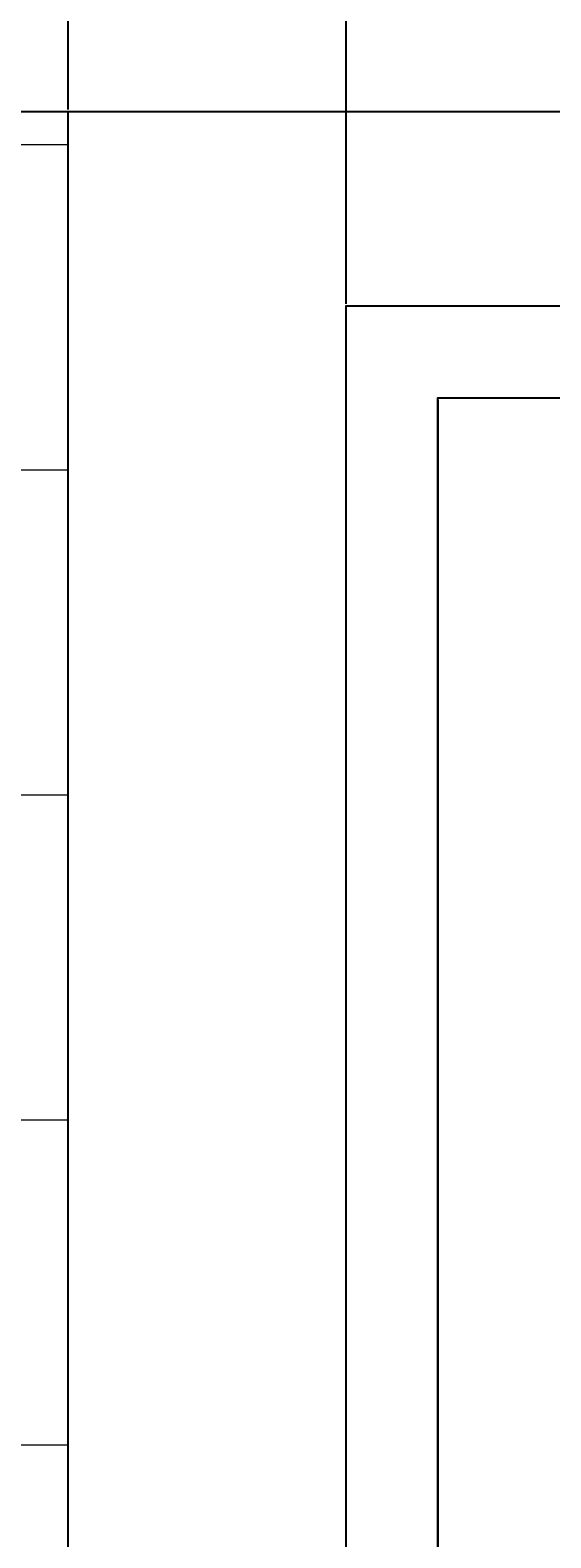
# Model space of a CAD drawing. Units: inches. Extents: x 37 to 824, y -700 to 234.
# Tile 16 of 77: x 298 to 315, y -536 to -487. Entities that reach past the tile are written whole.
import ezdxf

# ---------------------------------------------------------------- set-up
doc = ezdxf.new("R2010")
doc.units = ezdxf.units.IN
doc.header["$MEASUREMENT"] = 0
for name, color, linetype, lineweight in [('A-ANNO-DIMS', 2, 'Continuous', 18), ('A-DOOR', 4, 'Continuous', 25), ('A-ELEV', 3, 'Continuous', 25), ('A-ELEV-PATT', 8, 'Continuous', 13)]:
    doc.layers.add(name, color=color, linetype=linetype, lineweight=lineweight)
doc.styles.get("Standard").update_dxf_attribs({"font": 'arial.ttf'})
doc.dimstyles.get("Standard").update_dxf_attribs({"dimtxt": 0.18, "dimasz": 0.18, "dimexe": 0.18, "dimexo": 0.0625, "dimgap": 0.09, "dimtad": 0, "dimtih": 1, "dimtoh": 1, "dimdec": 1, "dimzin": 0, "dimdsep": 46, "dimlunit": 4, "dimtxsty": 'Standard', "dimcen": 0.09, "dimadec": 0, "dimazin": 0, "dimtfac": 1, "dimtdec": 1, "dimtofl": 0, "dimtmove": 0, "dimatfit": 3, "dimfxl": 1, "dimtolj": 1, "dimtzin": 0, "dimarcsym": 0})

# ---------------------------------------------------------------- blocks, each defined once
blk = doc.blocks.new('*U9')
blk.add_lwpolyline([(3.124, 0.013), (0.124, 0.013), (0.124, 84.013), (40.124, 84.013), (40.124, 0.013), (37.124, 0.013)])
blk.add_lwpolyline([(37.124, 80.99), (37.124, 0.013), (3.124, 0.013), (3.124, 80.99)], close=True)
blk = doc.blocks.new('*D31')
at = {"layer": 'A-ANNO-DIMS', "color": 0, "lineweight": -2, "ltscale": 0.5, "transparency": 16777216}
for p, q in [((255.14, -489.627), (449.772, -489.627)), ((449.592, -495.627), (449.592, -510.537)), ((449.592, -531.627), (449.592, -516.717)), ((255.14, -537.627), (449.772, -537.627))]:
    blk.add_line(p, q, dxfattribs=at)
at = {"layer": 'A-ANNO-DIMS', "color": 0, "ltscale": 0.5, "transparency": 16777216}
for points in [[(448.592, -495.627), (450.592, -495.627), (449.592, -489.627)], [(448.592, -531.627), (450.592, -531.627), (449.592, -537.627)]]:
    blk.add_solid(points, dxfattribs=at)
at = {"layer": 'Defpoints', "color": 0, "ltscale": 0.5, "transparency": 16777216}
for p in [(255.077, -489.627), (449.592, -489.627), (255.077, -537.627)]:
    blk.add_point(p, dxfattribs=at)
at = {"layer": 'A-ANNO-DIMS', "color": 0, "ltscale": 0.5, "transparency": 16777216, "insert": (449.592, -513.627), "char_height": 6, "attachment_point": 5}
blk.add_mtext("\\A1;4'", dxfattribs=at)
blk = doc.blocks.new('*D98')
at = {"layer": 'A-ANNO-DIMS', "color": 0, "lineweight": -2, "ltscale": 0.5, "transparency": 16777216}
for p, q in [((299.077, -489.565), (299.077, -378.38)), ((308.196, -495.944), (308.196, -378.38)), ((299.257, -378.56), (303.307, -378.56)), ((308.016, -378.56), (303.966, -378.56))]:
    blk.add_line(p, q, dxfattribs=at)
at = {"layer": 'A-ANNO-DIMS', "color": 0, "ltscale": 0.5, "transparency": 16777216}
for points in [[(299.257, -378.53), (299.257, -378.59), (299.077, -378.56)], [(308.016, -378.53), (308.016, -378.59), (308.196, -378.56)]]:
    blk.add_solid(points, dxfattribs=at)
at = {"layer": 'Defpoints', "color": 0, "ltscale": 0.5, "transparency": 16777216}
for p in [(308.196, -378.56), (299.077, -489.627), (308.196, -496.007)]:
    blk.add_point(p, dxfattribs=at)
at = {"layer": 'A-ANNO-DIMS', "color": 0, "ltscale": 0.5, "transparency": 16777216, "insert": (303.636, -378.56), "char_height": 0.18, "attachment_point": 5}
blk.add_mtext('\\A1;0\'-9"', dxfattribs=at)
blk = doc.blocks.new('*D99')
at = {"layer": 'A-ANNO-DIMS', "color": 0, "lineweight": -2, "ltscale": 0.5, "transparency": 16777216}
for p, q in [((308.196, -495.944), (308.196, -378.38)), ((348.196, -495.944), (348.196, -378.38)), ((308.376, -378.56), (327.866, -378.56)), ((348.016, -378.56), (328.525, -378.56))]:
    blk.add_line(p, q, dxfattribs=at)
at = {"layer": 'A-ANNO-DIMS', "color": 0, "ltscale": 0.5, "transparency": 16777216}
for points in [[(308.376, -378.53), (308.376, -378.59), (308.196, -378.56)], [(348.016, -378.53), (348.016, -378.59), (348.196, -378.56)]]:
    blk.add_solid(points, dxfattribs=at)
at = {"layer": 'Defpoints', "color": 0, "ltscale": 0.5, "transparency": 16777216}
for p in [(348.196, -378.56), (308.196, -496.007), (348.196, -496.007)]:
    blk.add_point(p, dxfattribs=at)
at = {"layer": 'A-ANNO-DIMS', "color": 0, "ltscale": 0.5, "transparency": 16777216, "insert": (328.196, -378.56), "char_height": 0.18, "attachment_point": 5}
blk.add_mtext('\\A1;3\'-4"', dxfattribs=at)
blk = doc.blocks.new('*D102')
at = {"layer": 'A-ANNO-DIMS', "color": 0, "lineweight": -2, "ltscale": 0.5, "transparency": 16777216}
for p, q in [((311.196, -499.092), (311.196, -699.594)), ((345.196, -499.092), (345.196, -699.594)), ((311.376, -699.414), (327.795, -699.414)), ((345.016, -699.414), (328.596, -699.414))]:
    blk.add_line(p, q, dxfattribs=at)
at = {"layer": 'A-ANNO-DIMS', "color": 0, "ltscale": 0.5, "transparency": 16777216}
for points in [[(311.376, -699.384), (311.376, -699.444), (311.196, -699.414)], [(345.016, -699.384), (345.016, -699.444), (345.196, -699.414)]]:
    blk.add_solid(points, dxfattribs=at)
at = {"layer": 'Defpoints', "color": 0, "ltscale": 0.5, "transparency": 16777216}
for p in [(311.196, -499.03), (345.196, -499.03), (345.196, -699.414)]:
    blk.add_point(p, dxfattribs=at)
at = {"layer": 'A-ANNO-DIMS', "color": 0, "ltscale": 0.5, "transparency": 16777216, "insert": (328.196, -699.414), "char_height": 0.18, "attachment_point": 5}
blk.add_mtext('\\A1;2\'-10"', dxfattribs=at)

msp = doc.modelspace()

# ---------------------------------------------------------------- hatches: boundary and pattern name
at = {"layer": 'A-ELEV-PATT', "ltscale": 0.5}
h = msp.add_hatch(dxfattribs=at)
h.set_pattern_fill('AR-BRSTD', color=256, scale=4)
h.paths.add_polyline_path([(299.077, -489.627), (358.132, -489.627), (358.132, -585.627), (428.077, -585.627), (428.077, -465.627), (161.077, -465.627), (161.077, -585.627), (299.077, -585.627)])
h.paths.add_polyline_path([(205.077, -537.627), (205.077, -489.627), (255.077, -489.627), (255.077, -537.627)], flags=16)

# ---------------------------------------------------------------- linework, layer by layer
at = {"layer": 'A-ELEV', "ltscale": 0.5}
msp.add_lwpolyline([(299.077, -489.627), (358.132, -489.627), (358.132, -585.627), (299.077, -585.627)], close=True, dxfattribs=at)

# ---------------------------------------------------------------- block references
at = {"layer": 'A-DOOR'}
msp.add_blockref('*U9', (308.072, -580.019), dxfattribs=at)

# ---------------------------------------------------------------- dimensions: what is measured, and where the dimension line sits
at = {"layer": 'A-ANNO-DIMS', "ltscale": 0.5}
for base, p1, p2, picture, middle in [((308.196, -378.56), (299.077, -489.627), (308.196, -496.007), '*D98', (303.636, -378.56)), ((348.196, -378.56), (308.196, -496.007), (348.196, -496.007), '*D99', (328.196, -378.56)), ((345.196, -699.414), (311.196, -499.03), (345.196, -499.03), '*D102', (328.196, -699.414))]:
    dim = msp.add_linear_dim(base=base, p1=p1, p2=p2, dimstyle='Standard', override={"dimdec": 1, "dimlfac": 1, "dimrnd": 0, "dimzin": 1, "dimdsep": 46, "dimlunit": 4, "dimfrac": 2}, dxfattribs=at)
    dim.commit()
    dim.dimension.update_dxf_attribs({"geometry": picture, "text_midpoint": middle})
dim = msp.add_linear_dim(base=(449.592, -489.627), p1=(255.077, -537.627), p2=(255.077, -489.627), angle=90, dimstyle='Standard', override={"dimtxt": 6, "dimasz": 6, "dimclrd": 0, "dimclre": 0, "dimclrt": 0}, dxfattribs=at)
dim.commit()
dim.dimension.update_dxf_attribs({"geometry": '*D31', "text_midpoint": (449.592, -513.627)})

doc.saveas('drawing.dxf')
